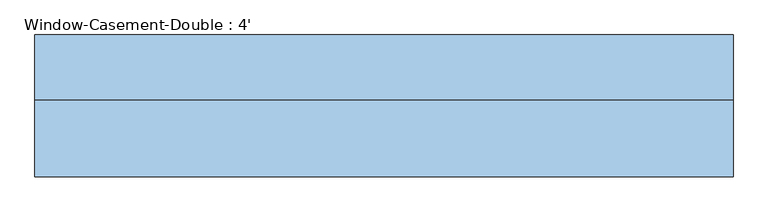
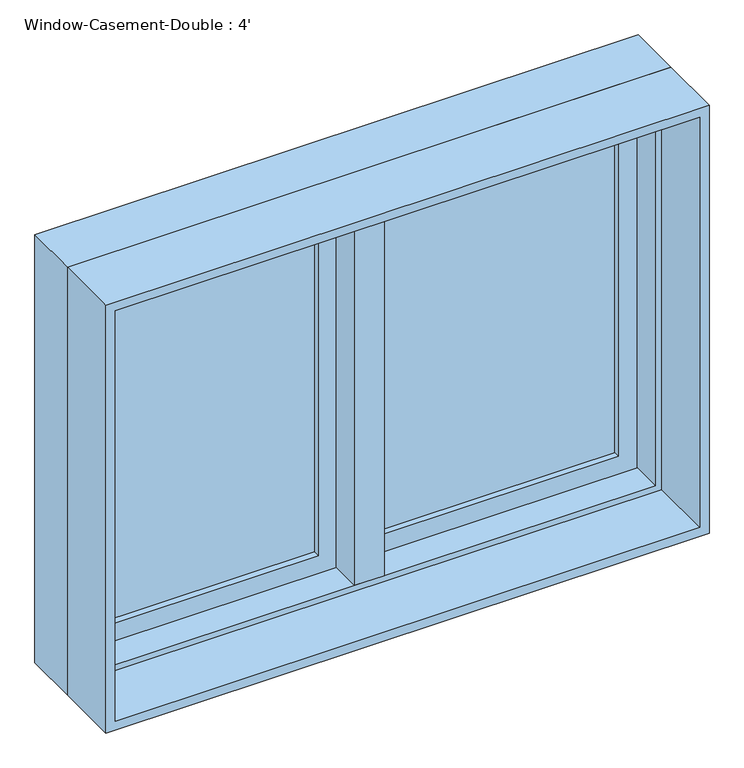
"""IFC4 building model written with IfcOpenShell, lengths in millimetres: window geometry, Window-Casement-Double : 4'."""

from ifc_helpers import new_model, si_unit, frame, origin, place, context, project, spatial, polyline, outline, extrude, faceted_brep, source, transform, mapped, element, save


def window_casement_double_4_c19c33cb(model_context):
    return source(origin(), model_context, "Body", "SolidModel", [
        faceted_brep([(9.525, 133.35, 1816.1), (-9.525, 133.35, 1816.1), (-9.525, 82.55, 1816.1), (9.525, 82.55, 1816.1), (9.525, 133.35, 927.1), (9.525, 82.55, 927.1), (-9.525, 82.55, 927.1), (-9.525, 133.35, 927.1), (-9.525, 82.55, 946.15), (-9.525, 82.55, 1797.05), (-30.1625, 82.55, 946.15), (-30.1625, 82.55, 1797.05), (-30.1625, 19.05, 946.15), (-30.1625, 19.05, 1797.05), (30.1625, 19.05, 946.15), (30.1625, 19.05, 1797.05), (30.1625, 82.55, 946.15), (30.1625, 82.55, 1797.05), (9.525, 82.55, 946.15), (9.525, 82.55, 1797.05)], [[[0, 1, 2, 3]], [[4, 5, 6, 7]], [[1, 0, 4, 7]], [[2, 1, 7, 6, 8, 9]], [[9, 8, 10, 11]], [[11, 10, 12, 13]], [[13, 12, 14, 15]], [[15, 14, 16, 17]], [[17, 16, 18, 19]], [[0, 3, 19, 18, 5, 4]], [[18, 8, 6, 5]], [[9, 19, 3, 2]], [[8, 18, 16, 14, 12, 10]], [[19, 9, 11, 13, 15, 17]]]),
        extrude(outline(polyline([(-66.675, 114.3), (-66.675, 107.95), (-539.75, 107.95), (-539.75, 114.3), (-66.675, 114.3)])), frame((0.0, 0.0, 984.25), z_axis=(0.0, 0.0, 1.0), x_axis=(1.0, 0.0, 0.0)), (0.0, 0.0, 1.0), 774.7),
        extrude(outline(polyline([(-539.75, 95.25), (-539.75, 101.6), (-66.675, 101.6), (-66.675, 95.25), (-539.75, 95.25)])), frame((0.0, 0.0, 984.25), z_axis=(0.0, 0.0, 1.0), x_axis=(1.0, 0.0, 0.0)), (0.0, 0.0, 1.0), 774.7),
        extrude(outline(polyline([(539.75, 114.3), (539.75, 107.95), (66.675, 107.95), (66.675, 114.3), (539.75, 114.3)])), frame((0.0, 0.0, 984.25), z_axis=(0.0, 0.0, 1.0), x_axis=(1.0, 0.0, 0.0)), (0.0, 0.0, 1.0), 774.7),
        extrude(outline(polyline([(66.675, 95.25), (66.675, 101.6), (539.75, 101.6), (539.75, 95.25), (66.675, 95.25)])), frame((0.0, 0.0, 984.25), z_axis=(0.0, 0.0, 1.0), x_axis=(1.0, 0.0, 0.0)), (0.0, 0.0, 1.0), 774.7),
        extrude(outline(polyline([(1816.1, -596.9), (927.1, -596.9), (927.1, -9.525), (1816.1, -9.525), (1816.1, -596.9)]), holes=[polyline([(1758.95, -66.675), (984.25, -66.675), (984.25, -539.75), (1758.95, -539.75), (1758.95, -66.675)])]), frame((0.0, 82.55, 0.0), z_axis=(0.0, 1.0, 0.0), x_axis=(0.0, 0.0, 1.0)), (0.0, 0.0, 1.0), 44.45),
        extrude(outline(polyline([(927.1, 596.9), (1816.1, 596.9), (1816.1, 9.525), (927.1, 9.525), (927.1, 596.9)]), holes=[polyline([(984.25, 66.675), (1758.95, 66.675), (1758.95, 539.75), (984.25, 539.75), (984.25, 66.675)])]), frame((0.0, 82.55, 0.0), z_axis=(0.0, 1.0, 0.0), x_axis=(0.0, 0.0, 1.0)), (0.0, 0.0, 1.0), 44.45),
        extrude(outline(polyline([(1828.8, -609.6), (914.4, -609.6), (914.4, 609.6), (1828.8, 609.6), (1828.8, -609.6)]), holes=[polyline([(1809.75, 590.55), (933.45, 590.55), (933.45, -590.55), (1809.75, -590.55), (1809.75, 590.55)])]), frame((0.0, -114.3, 0.0), z_axis=(0.0, 1.0, 0.0), x_axis=(0.0, 0.0, 1.0)), (0.0, 0.0, 1.0), 133.35),
        faceted_brep([(577.85, 82.55, 1797.05), (577.85, 19.05, 1797.05), (-577.85, 19.05, 1797.05), (-577.85, 82.55, 1797.05), (596.9, 133.35, 1816.1), (596.9, 82.55, 1816.1), (-596.9, 82.55, 1816.1), (-596.9, 133.35, 1816.1), (609.6, 19.05, 1828.8), (609.6, 133.35, 1828.8), (-609.6, 133.35, 1828.8), (-609.6, 19.05, 1828.8), (-577.85, 19.05, 946.15), (-577.85, 82.55, 946.15), (-596.9, 82.55, 927.1), (-596.9, 133.35, 927.1), (-609.6, 133.35, 914.4), (-609.6, 19.05, 914.4), (577.85, 19.05, 946.15), (577.85, 82.55, 946.15), (596.9, 82.55, 927.1), (596.9, 133.35, 927.1), (609.6, 133.35, 914.4), (609.6, 19.05, 914.4)], [[[0, 1, 2, 3]], [[4, 5, 6, 7]], [[8, 9, 10, 11]], [[3, 2, 12, 13]], [[7, 6, 14, 15]], [[11, 10, 16, 17]], [[13, 12, 18, 19]], [[15, 14, 20, 21]], [[17, 16, 22, 23]], [[11, 17, 23, 8], [1, 18, 12, 2]], [[19, 18, 1, 0]], [[5, 20, 14, 6], [3, 13, 19, 0]], [[21, 20, 5, 4]], [[23, 22, 9, 8]], [[9, 22, 16, 10], [7, 15, 21, 4]]]),
    ])


if __name__ == "__main__":
    model = new_model("IFC4")
    model_context = context("Model", 3, world=origin())
    ifc_project = project(units=[si_unit("LENGTHUNIT", "METRE", prefix="MILLI")], contexts=[model_context])
    site = spatial("IfcSite", under=ifc_project)
    building = spatial("IfcBuilding", under=site)
    placement = place(None, origin())
    window_casement_double_4_shape = window_casement_double_4_c19c33cb(model_context)
    element("IfcWindow", 1, ObjectType="Window-Casement-Double : 4'", at=placement, inside=building, context=model_context, shape_type="MappedRepresentation", body=[
        mapped(window_casement_double_4_shape, transform((0.0, 0.0, 0.0), x_axis=(1.0, 0.0, 0.0), y_axis=(0.0, 1.0, 0.0), z_axis=(0.0, 0.0, 1.0))),
    ])
    save(model, "model.ifc")

# Revit data of these elements
# Type "Window-Casement-Double : 4'"
#   Type Mark = "18"
#   Fire Rating = "0.5h"
#   Assembly Code = "B2020100"
#   Analytic Construction = "Double glazing - domestic"
#   Frame Extension [instance default] = 0' - 0 1/4"
#   Window Inset [instance default] = 0' - 0"
#   Wall Thickness [instance default] = 0' - 6"
#   Interior Wall Closure [instance default] = 0' - 2 1/4"
#   Half Width = 2' - 0"
#   Visual Light Transmittance = 0.81
#   Thermal Resistance (R) = 1.8146 (h·ft²·°F)/BTU
#   Solar Heat Gain Coefficient = 0.76
#   Rough Width = 4' - 0 1/2"
#   Rough Height = 3' - 0 1/2"
#   Height = 3' - 0"
#   Heat Transfer Coefficient (U) = 0.5511 BTU/(h·ft²·°F)
#   Exterior Wall Closure [instance default] = 0' - 1 1/4"
#   Extension Jamb [instance default] = 0' - 2 1/4"
#   Default Sill Height = 3' - 0"
#   Width = 4' - 0"
#   Muntin Visibility = yes
#   Interior Trim Visibility [instance default] = yes
#   Exterior Trim Visibility [instance default] = yes
#   Extension Jamb Visibility [instance default] = yes
#   Interior Trim Material = Wood - Stained
#   Muntin Pattern = Muntin Pattern_2x2 : Muntin Pattern_2x2
#   Interior Trim = Trim-Window-Interior-Flat : Picture Frame
#   Interior Frame Material = Wood - Stained
#   Glass Panel Material = Glass
#   Exterior Trim Material = Clad - White
#   Exterior Trim = Trim-Window-Exterior-Flat : with Sill
#   Exterior Frame Material = Clad - White
#   Wall Closure = (empty or 0)
# Element 1 (IfcWindow, "Window-Casement-Double : 4'")
#   Wall Thickness = 0' - 9"
#   Extension Jamb = 0' - 5 1/4"
#   Materials on its faces: "Wood - Stained", "Glass", "Clad - White"
# Materials
#   "Wood - Stained": class "Wood", colour RGB 224 178 126, transparency 0, Cost = 0
#   "Glass": class "Glass", colour RGB 0 128 192, transparency 0.75, Description = "Soda Lime Glass", Cost = 0
#   "Clad - White": class "Wood", colour RGB 242 242 238, transparency 0, Cost = 0
